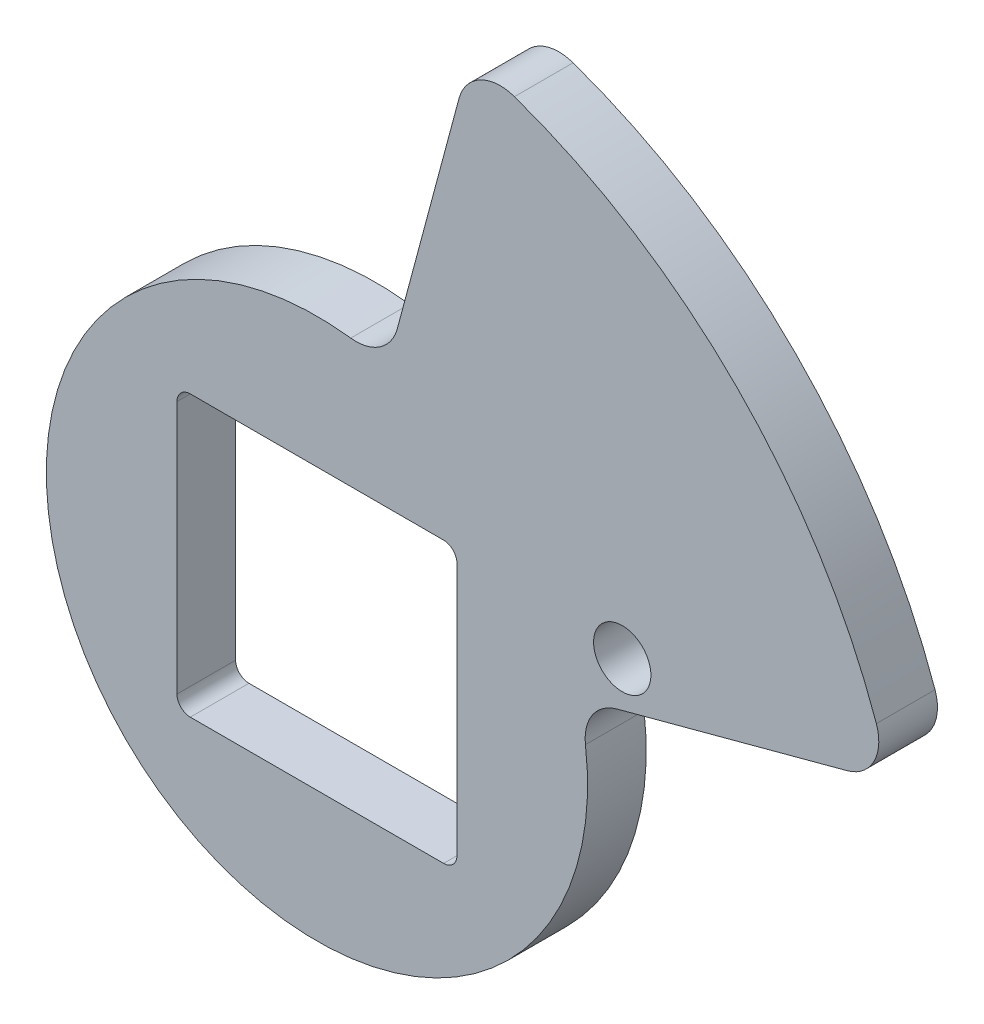
ISO-10303-21;
HEADER;
FILE_DESCRIPTION(('STEP AP214'),'2;1');
FILE_NAME('part.step','',(''),(''),'','','');
FILE_SCHEMA(('AUTOMOTIVE_DESIGN { 1 0 10303 214 1 1 1 1 }'));
ENDSEC;
DATA;
#1=APPLICATION_CONTEXT('core data for automotive mechanical design processes');
#2=APPLICATION_PROTOCOL_DEFINITION('international standard','automotive_design',2000,#1);
#3=PRODUCT_CONTEXT('',#1,'mechanical');
#4=PRODUCT('Part','Part','',(#3));
#5=PRODUCT_RELATED_PRODUCT_CATEGORY('part','',(#4));
#6=PRODUCT_DEFINITION_FORMATION('','',#4);
#7=PRODUCT_DEFINITION_CONTEXT('part definition',#1,'design');
#8=PRODUCT_DEFINITION('design','',#6,#7);
#9=PRODUCT_DEFINITION_SHAPE('','',#8);
#10=(LENGTH_UNIT() NAMED_UNIT(*) SI_UNIT(.MILLI.,.METRE.));
#11=(NAMED_UNIT(*) PLANE_ANGLE_UNIT() SI_UNIT($,.RADIAN.));
#12=(NAMED_UNIT(*) SI_UNIT($,.STERADIAN.) SOLID_ANGLE_UNIT());
#13=UNCERTAINTY_MEASURE_WITH_UNIT(LENGTH_MEASURE(1.E-05),#10,'distance_accuracy_value','');
#14=(GEOMETRIC_REPRESENTATION_CONTEXT(3) GLOBAL_UNCERTAINTY_ASSIGNED_CONTEXT((#13)) GLOBAL_UNIT_ASSIGNED_CONTEXT((#10,
#11,#12)) REPRESENTATION_CONTEXT('',''));
#15=CARTESIAN_POINT('',(0.,0.,0.));
#16=DIRECTION('',(0.,0.,1.));
#17=DIRECTION('',(1.,0.,0.));
#18=AXIS2_PLACEMENT_3D('',#15,#16,#17);
#19=CARTESIAN_POINT('',(2.93463155457416,23.316044639666,4.4));
#20=DIRECTION('',(0.,0.,-1.));
#21=DIRECTION('',(-1.,0.,0.));
#22=AXIS2_PLACEMENT_3D('',#19,#20,#21);
#23=CYLINDRICAL_SURFACE('',#22,3.20000000000004);
#24=CARTESIAN_POINT('',(2.93463155457416,23.316044639666,0.));
#25=DIRECTION('',(0.,0.,-1.));
#26=DIRECTION('',(1.,0.,0.));
#27=AXIS2_PLACEMENT_3D('',#24,#25,#26);
#28=CIRCLE('',#27,3.20000000000004);
#29=CARTESIAN_POINT('',(6.02559419869927,22.487823695338,0.));
#30=VERTEX_POINT('',#29);
#31=CARTESIAN_POINT('',(2.53502215139811,20.1410938802221,0.));
#32=VERTEX_POINT('',#31);
#33=EDGE_CURVE('E224',#30,#32,#28,.T.);
#34=ORIENTED_EDGE('',*,*,#33,.T.);
#35=DIRECTION('',(0.,0.,-1.));
#36=VECTOR('',#35,1.);
#37=CARTESIAN_POINT('',(2.53502215139811,20.1410938802221,4.4));
#38=LINE('',#37,#36);
#39=CARTESIAN_POINT('',(2.53502215139811,20.1410938802221,4.4));
#40=VERTEX_POINT('',#39);
#41=EDGE_CURVE('E259',#40,#32,#38,.T.);
#42=ORIENTED_EDGE('',*,*,#41,.F.);
#43=CARTESIAN_POINT('',(2.93463155457416,23.316044639666,4.4));
#44=DIRECTION('',(0.,0.,-1.));
#45=DIRECTION('',(1.,0.,0.));
#46=AXIS2_PLACEMENT_3D('',#43,#44,#45);
#47=CIRCLE('',#46,3.20000000000004);
#48=CARTESIAN_POINT('',(6.02559419869927,22.487823695338,4.4));
#49=VERTEX_POINT('',#48);
#50=EDGE_CURVE('E204',#49,#40,#47,.T.);
#51=ORIENTED_EDGE('',*,*,#50,.F.);
#52=DIRECTION('',(0.,0.,-1.));
#53=VECTOR('',#52,1.);
#54=CARTESIAN_POINT('',(6.02559419869927,22.487823695338,4.4));
#55=LINE('',#54,#53);
#56=EDGE_CURVE('E225',#49,#30,#55,.T.);
#57=ORIENTED_EDGE('',*,*,#56,.T.);
#58=EDGE_LOOP('',(#34,#42,#51,#57));
#59=FACE_BOUND('',#58,.T.);
#60=ADVANCED_FACE('F39',(#59),#23,.F.);
#61=CARTESIAN_POINT('',(0.,0.,4.4));
#62=DIRECTION('',(0.,0.,-1.));
#63=DIRECTION('',(-1.,0.,0.));
#64=AXIS2_PLACEMENT_3D('',#61,#62,#63);
#65=CYLINDRICAL_SURFACE('',#64,20.3);
#66=CARTESIAN_POINT('',(0.,0.,0.));
#67=DIRECTION('',(0.,0.,1.));
#68=DIRECTION('',(1.,0.,0.));
#69=AXIS2_PLACEMENT_3D('',#66,#67,#68);
#70=CIRCLE('',#69,20.3);
#71=CARTESIAN_POINT('',(20.1410938802221,2.5350221513982,0.));
#72=VERTEX_POINT('',#71);
#73=EDGE_CURVE('E227',#32,#72,#70,.T.);
#74=ORIENTED_EDGE('',*,*,#73,.T.);
#75=DIRECTION('',(0.,0.,-1.));
#76=VECTOR('',#75,1.);
#77=CARTESIAN_POINT('',(20.1410938802221,2.5350221513982,4.4));
#78=LINE('',#77,#76);
#79=CARTESIAN_POINT('',(20.1410938802221,2.5350221513982,4.4));
#80=VERTEX_POINT('',#79);
#81=EDGE_CURVE('E258',#80,#72,#78,.T.);
#82=ORIENTED_EDGE('',*,*,#81,.F.);
#83=CARTESIAN_POINT('',(0.,0.,4.4));
#84=DIRECTION('',(0.,0.,1.));
#85=DIRECTION('',(1.,0.,0.));
#86=AXIS2_PLACEMENT_3D('',#83,#84,#85);
#87=CIRCLE('',#86,20.3);
#88=EDGE_CURVE('E210',#40,#80,#87,.T.);
#89=ORIENTED_EDGE('',*,*,#88,.F.);
#90=ORIENTED_EDGE('',*,*,#41,.T.);
#91=EDGE_LOOP('',(#74,#82,#89,#90));
#92=FACE_BOUND('',#91,.T.);
#93=ADVANCED_FACE('F311',(#92),#65,.T.);
#94=CARTESIAN_POINT('',(23.316044639666,2.93463155457426,4.4));
#95=DIRECTION('',(0.,0.,-1.));
#96=DIRECTION('',(-1.,0.,0.));
#97=AXIS2_PLACEMENT_3D('',#94,#95,#96);
#98=CYLINDRICAL_SURFACE('',#97,3.2);
#99=CARTESIAN_POINT('',(23.316044639666,2.93463155457426,0.));
#100=DIRECTION('',(0.,0.,-1.));
#101=DIRECTION('',(1.,0.,0.));
#102=AXIS2_PLACEMENT_3D('',#99,#100,#101);
#103=CIRCLE('',#102,3.2);
#104=CARTESIAN_POINT('',(22.4878236953379,6.02559419869928,0.));
#105=VERTEX_POINT('',#104);
#106=EDGE_CURVE('E229',#72,#105,#103,.T.);
#107=ORIENTED_EDGE('',*,*,#106,.T.);
#108=DIRECTION('',(0.,0.,-1.));
#109=VECTOR('',#108,1.);
#110=CARTESIAN_POINT('',(22.4878236953379,6.02559419869928,4.4));
#111=LINE('',#110,#109);
#112=CARTESIAN_POINT('',(22.4878236953379,6.02559419869928,4.4));
#113=VERTEX_POINT('',#112);
#114=EDGE_CURVE('E251',#113,#105,#111,.T.);
#115=ORIENTED_EDGE('',*,*,#114,.F.);
#116=CARTESIAN_POINT('',(23.316044639666,2.93463155457426,4.4));
#117=DIRECTION('',(0.,0.,-1.));
#118=DIRECTION('',(1.,0.,0.));
#119=AXIS2_PLACEMENT_3D('',#116,#117,#118);
#120=CIRCLE('',#119,3.2);
#121=EDGE_CURVE('E209',#80,#113,#120,.T.);
#122=ORIENTED_EDGE('',*,*,#121,.F.);
#123=ORIENTED_EDGE('',*,*,#81,.T.);
#124=EDGE_LOOP('',(#107,#115,#122,#123));
#125=FACE_BOUND('',#124,.T.);
#126=ADVANCED_FACE('F318',(#125),#98,.F.);
#127=CARTESIAN_POINT('',(22.4878236953379,6.02559419869928,4.4));
#128=DIRECTION('',(-0.258819045102526,0.965925826289067,0.));
#129=DIRECTION('',(-0.965925826289067,-0.258819045102526,0.));
#130=AXIS2_PLACEMENT_3D('',#127,#128,#129);
#131=PLANE('',#130);
#132=DIRECTION('',(0.965925826289067,0.258819045102526,0.));
#133=VECTOR('',#132,1.);
#134=CARTESIAN_POINT('',(22.4878236953379,6.02559419869928,0.));
#135=LINE('',#134,#133);
#136=CARTESIAN_POINT('',(39.7728096244553,10.6570922195897,0.));
#137=VERTEX_POINT('',#136);
#138=EDGE_CURVE('E228',#105,#137,#135,.T.);
#139=ORIENTED_EDGE('',*,*,#138,.T.);
#140=DIRECTION('',(0.,0.,-1.));
#141=VECTOR('',#140,1.);
#142=CARTESIAN_POINT('',(39.7728096244553,10.6570922195897,4.4));
#143=LINE('',#142,#141);
#144=CARTESIAN_POINT('',(39.7728096244553,10.6570922195897,4.4));
#145=VERTEX_POINT('',#144);
#146=EDGE_CURVE('E246',#145,#137,#143,.T.);
#147=ORIENTED_EDGE('',*,*,#146,.F.);
#148=DIRECTION('',(0.965925826289067,0.258819045102526,0.));
#149=VECTOR('',#148,1.);
#150=CARTESIAN_POINT('',(22.4878236953379,6.02559419869928,4.4));
#151=LINE('',#150,#149);
#152=EDGE_CURVE('E215',#113,#145,#151,.T.);
#153=ORIENTED_EDGE('',*,*,#152,.F.);
#154=ORIENTED_EDGE('',*,*,#114,.T.);
#155=EDGE_LOOP('',(#139,#147,#153,#154));
#156=FACE_BOUND('',#155,.T.);
#157=ADVANCED_FACE('F355',(#156),#131,.F.);
#158=CARTESIAN_POINT('',(38.9445886801272,13.7480548637146,4.4));
#159=DIRECTION('',(0.,0.,-1.));
#160=DIRECTION('',(-1.,0.,0.));
#161=AXIS2_PLACEMENT_3D('',#158,#159,#160);
#162=CYLINDRICAL_SURFACE('',#161,3.19999999999996);
#163=CARTESIAN_POINT('',(38.9445886801272,13.7480548637146,0.));
#164=DIRECTION('',(0.,0.,1.));
#165=DIRECTION('',(1.,0.,0.));
#166=AXIS2_PLACEMENT_3D('',#163,#164,#165);
#167=CIRCLE('',#166,3.19999999999996);
#168=CARTESIAN_POINT('',(41.9620870766504,14.8132794536393,0.));
#169=VERTEX_POINT('',#168);
#170=EDGE_CURVE('E235',#137,#169,#167,.T.);
#171=ORIENTED_EDGE('',*,*,#170,.T.);
#172=DIRECTION('',(0.,0.,-1.));
#173=VECTOR('',#172,1.);
#174=CARTESIAN_POINT('',(41.9620870766504,14.8132794536393,4.4));
#175=LINE('',#174,#173);
#176=CARTESIAN_POINT('',(41.9620870766504,14.8132794536393,4.4));
#177=VERTEX_POINT('',#176);
#178=EDGE_CURVE('E250',#177,#169,#175,.T.);
#179=ORIENTED_EDGE('',*,*,#178,.F.);
#180=CARTESIAN_POINT('',(38.9445886801272,13.7480548637146,4.4));
#181=DIRECTION('',(0.,0.,1.));
#182=DIRECTION('',(1.,0.,0.));
#183=AXIS2_PLACEMENT_3D('',#180,#181,#182);
#184=CIRCLE('',#183,3.19999999999996);
#185=EDGE_CURVE('E212',#145,#177,#184,.T.);
#186=ORIENTED_EDGE('',*,*,#185,.F.);
#187=ORIENTED_EDGE('',*,*,#146,.T.);
#188=EDGE_LOOP('',(#171,#179,#186,#187));
#189=FACE_BOUND('',#188,.T.);
#190=ADVANCED_FACE('F346',(#189),#162,.T.);
#191=CARTESIAN_POINT('',(0.,0.,4.4));
#192=DIRECTION('',(0.,0.,-1.));
#193=DIRECTION('',(-1.,0.,0.));
#194=AXIS2_PLACEMENT_3D('',#191,#192,#193);
#195=CYLINDRICAL_SURFACE('',#194,44.5);
#196=CARTESIAN_POINT('',(0.,0.,0.));
#197=DIRECTION('',(0.,0.,1.));
#198=DIRECTION('',(1.,0.,0.));
#199=AXIS2_PLACEMENT_3D('',#196,#197,#198);
#200=CIRCLE('',#199,44.5);
#201=CARTESIAN_POINT('',(14.8132794536391,41.9620870766505,0.));
#202=VERTEX_POINT('',#201);
#203=EDGE_CURVE('E234',#169,#202,#200,.T.);
#204=ORIENTED_EDGE('',*,*,#203,.T.);
#205=DIRECTION('',(0.,0.,-1.));
#206=VECTOR('',#205,1.);
#207=CARTESIAN_POINT('',(14.8132794536391,41.9620870766505,4.4));
#208=LINE('',#207,#206);
#209=CARTESIAN_POINT('',(14.8132794536391,41.9620870766505,4.4));
#210=VERTEX_POINT('',#209);
#211=EDGE_CURVE('E241',#210,#202,#208,.T.);
#212=ORIENTED_EDGE('',*,*,#211,.F.);
#213=CARTESIAN_POINT('',(0.,0.,4.4));
#214=DIRECTION('',(0.,0.,1.));
#215=DIRECTION('',(1.,0.,0.));
#216=AXIS2_PLACEMENT_3D('',#213,#214,#215);
#217=CIRCLE('',#216,44.5);
#218=EDGE_CURVE('E216',#177,#210,#217,.T.);
#219=ORIENTED_EDGE('',*,*,#218,.F.);
#220=ORIENTED_EDGE('',*,*,#178,.T.);
#221=EDGE_LOOP('',(#204,#212,#219,#220));
#222=FACE_BOUND('',#221,.T.);
#223=ADVANCED_FACE('F343',(#222),#195,.T.);
#224=CARTESIAN_POINT('',(13.7480548637145,38.9445886801273,4.4));
#225=DIRECTION('',(0.,0.,-1.));
#226=DIRECTION('',(-1.,0.,0.));
#227=AXIS2_PLACEMENT_3D('',#224,#225,#226);
#228=CYLINDRICAL_SURFACE('',#227,3.2);
#229=CARTESIAN_POINT('',(13.7480548637145,38.9445886801273,0.));
#230=DIRECTION('',(0.,0.,1.));
#231=DIRECTION('',(1.,0.,0.));
#232=AXIS2_PLACEMENT_3D('',#229,#230,#231);
#233=CIRCLE('',#232,3.2);
#234=CARTESIAN_POINT('',(10.6570922195894,39.7728096244553,0.));
#235=VERTEX_POINT('',#234);
#236=EDGE_CURVE('E237',#202,#235,#233,.T.);
#237=ORIENTED_EDGE('',*,*,#236,.T.);
#238=DIRECTION('',(0.,0.,-1.));
#239=VECTOR('',#238,1.);
#240=CARTESIAN_POINT('',(10.6570922195894,39.7728096244553,4.4));
#241=LINE('',#240,#239);
#242=CARTESIAN_POINT('',(10.6570922195894,39.7728096244553,4.4));
#243=VERTEX_POINT('',#242);
#244=EDGE_CURVE('E242',#243,#235,#241,.T.);
#245=ORIENTED_EDGE('',*,*,#244,.F.);
#246=CARTESIAN_POINT('',(13.7480548637145,38.9445886801273,4.4));
#247=DIRECTION('',(0.,0.,1.));
#248=DIRECTION('',(1.,0.,0.));
#249=AXIS2_PLACEMENT_3D('',#246,#247,#248);
#250=CIRCLE('',#249,3.2);
#251=EDGE_CURVE('E217',#210,#243,#250,.T.);
#252=ORIENTED_EDGE('',*,*,#251,.F.);
#253=ORIENTED_EDGE('',*,*,#211,.T.);
#254=EDGE_LOOP('',(#237,#245,#252,#253));
#255=FACE_BOUND('',#254,.T.);
#256=ADVANCED_FACE('F339',(#255),#228,.T.);
#257=CARTESIAN_POINT('',(6.02559419869927,22.487823695338,4.4));
#258=DIRECTION('',(0.96592582628907,-0.258819045102513,0.));
#259=DIRECTION('',(0.258819045102513,0.96592582628907,0.));
#260=AXIS2_PLACEMENT_3D('',#257,#258,#259);
#261=PLANE('',#260);
#262=DIRECTION('',(-0.258819045102513,-0.96592582628907,0.));
#263=VECTOR('',#262,1.);
#264=CARTESIAN_POINT('',(6.02559419869927,22.487823695338,0.));
#265=LINE('',#264,#263);
#266=EDGE_CURVE('E208',#235,#30,#265,.T.);
#267=ORIENTED_EDGE('',*,*,#266,.T.);
#268=ORIENTED_EDGE('',*,*,#56,.F.);
#269=DIRECTION('',(-0.258819045102513,-0.96592582628907,0.));
#270=VECTOR('',#269,1.);
#271=CARTESIAN_POINT('',(6.02559419869927,22.487823695338,4.4));
#272=LINE('',#271,#270);
#273=EDGE_CURVE('E219',#243,#49,#272,.T.);
#274=ORIENTED_EDGE('',*,*,#273,.F.);
#275=ORIENTED_EDGE('',*,*,#244,.T.);
#276=EDGE_LOOP('',(#267,#268,#274,#275));
#277=FACE_BOUND('',#276,.T.);
#278=ADVANCED_FACE('F337',(#277),#261,.F.);
#279=CARTESIAN_POINT('',(2.93463155457416,23.316044639666,4.4));
#280=DIRECTION('',(0.,0.,1.));
#281=DIRECTION('',(1.,0.,0.));
#282=AXIS2_PLACEMENT_3D('',#279,#280,#281);
#283=PLANE('',#282);
#284=CARTESIAN_POINT('',(-9.5,-9.5,4.4));
#285=DIRECTION('',(0.,0.,1.));
#286=DIRECTION('',(1.,0.,0.));
#287=AXIS2_PLACEMENT_3D('',#284,#285,#286);
#288=CIRCLE('',#287,0.999999999999999);
#289=CARTESIAN_POINT('',(-10.5,-9.49999999999999,4.4));
#290=VERTEX_POINT('',#289);
#291=CARTESIAN_POINT('',(-9.49999999999999,-10.5,4.4));
#292=VERTEX_POINT('',#291);
#293=EDGE_CURVE('E52',#290,#292,#288,.T.);
#294=ORIENTED_EDGE('',*,*,#293,.F.);
#295=DIRECTION('',(0.,-1.,0.));
#296=VECTOR('',#295,1.);
#297=CARTESIAN_POINT('',(-10.5,0.,4.4));
#298=LINE('',#297,#296);
#299=CARTESIAN_POINT('',(-10.5,9.49999999999999,4.4));
#300=VERTEX_POINT('',#299);
#301=EDGE_CURVE('E183',#300,#290,#298,.T.);
#302=ORIENTED_EDGE('',*,*,#301,.F.);
#303=CARTESIAN_POINT('',(-9.5,9.5,4.4));
#304=DIRECTION('',(0.,0.,1.));
#305=DIRECTION('',(1.,0.,0.));
#306=AXIS2_PLACEMENT_3D('',#303,#304,#305);
#307=CIRCLE('',#306,0.999999999999999);
#308=CARTESIAN_POINT('',(-9.49999999999999,10.5,4.4));
#309=VERTEX_POINT('',#308);
#310=EDGE_CURVE('E185',#309,#300,#307,.T.);
#311=ORIENTED_EDGE('',*,*,#310,.F.);
#312=DIRECTION('',(-1.,0.,0.));
#313=VECTOR('',#312,1.);
#314=CARTESIAN_POINT('',(9.49999999999999,10.5,4.4));
#315=LINE('',#314,#313);
#316=CARTESIAN_POINT('',(9.49999999999999,10.5,4.4));
#317=VERTEX_POINT('',#316);
#318=EDGE_CURVE('E179',#317,#309,#315,.T.);
#319=ORIENTED_EDGE('',*,*,#318,.F.);
#320=CARTESIAN_POINT('',(9.5,9.5,4.4));
#321=DIRECTION('',(0.,0.,1.));
#322=DIRECTION('',(1.,0.,0.));
#323=AXIS2_PLACEMENT_3D('',#320,#321,#322);
#324=CIRCLE('',#323,0.999999999999999);
#325=CARTESIAN_POINT('',(10.5,9.49999999999999,4.4));
#326=VERTEX_POINT('',#325);
#327=EDGE_CURVE('E174',#326,#317,#324,.T.);
#328=ORIENTED_EDGE('',*,*,#327,.F.);
#329=DIRECTION('',(0.,1.,0.));
#330=VECTOR('',#329,1.);
#331=CARTESIAN_POINT('',(10.5,-9.49999999999999,4.4));
#332=LINE('',#331,#330);
#333=CARTESIAN_POINT('',(10.5,-9.49999999999999,4.4));
#334=VERTEX_POINT('',#333);
#335=EDGE_CURVE('E172',#334,#326,#332,.T.);
#336=ORIENTED_EDGE('',*,*,#335,.F.);
#337=CARTESIAN_POINT('',(9.5,-9.5,4.4));
#338=DIRECTION('',(0.,0.,1.));
#339=DIRECTION('',(1.,0.,0.));
#340=AXIS2_PLACEMENT_3D('',#337,#338,#339);
#341=CIRCLE('',#340,1.);
#342=CARTESIAN_POINT('',(9.49999999999999,-10.5,4.4));
#343=VERTEX_POINT('',#342);
#344=EDGE_CURVE('E152',#343,#334,#341,.T.);
#345=ORIENTED_EDGE('',*,*,#344,.F.);
#346=DIRECTION('',(1.,0.,0.));
#347=VECTOR('',#346,1.);
#348=CARTESIAN_POINT('',(-9.49999999999999,-10.5,4.4));
#349=LINE('',#348,#347);
#350=EDGE_CURVE('E162',#292,#343,#349,.T.);
#351=ORIENTED_EDGE('',*,*,#350,.F.);
#352=EDGE_LOOP('',(#294,#302,#311,#319,#328,#336,#345,#351));
#353=FACE_BOUND('',#352,.T.);
#354=CARTESIAN_POINT('',(22.9,9.5,4.4));
#355=DIRECTION('',(0.,0.,1.));
#356=DIRECTION('',(1.,0.,0.));
#357=AXIS2_PLACEMENT_3D('',#354,#355,#356);
#358=CIRCLE('',#357,2.15);
#359=CARTESIAN_POINT('',(25.05,9.5,4.4));
#360=VERTEX_POINT('',#359);
#361=EDGE_CURVE('E203',#360,#360,#358,.T.);
#362=ORIENTED_EDGE('',*,*,#361,.F.);
#363=EDGE_LOOP('',(#362));
#364=FACE_BOUND('',#363,.T.);
#365=ORIENTED_EDGE('',*,*,#50,.T.);
#366=ORIENTED_EDGE('',*,*,#88,.T.);
#367=ORIENTED_EDGE('',*,*,#121,.T.);
#368=ORIENTED_EDGE('',*,*,#152,.T.);
#369=ORIENTED_EDGE('',*,*,#185,.T.);
#370=ORIENTED_EDGE('',*,*,#218,.T.);
#371=ORIENTED_EDGE('',*,*,#251,.T.);
#372=ORIENTED_EDGE('',*,*,#273,.T.);
#373=EDGE_LOOP('',(#365,#366,#367,#368,#369,#370,#371,#372));
#374=FACE_BOUND('',#373,.T.);
#375=ADVANCED_FACE('F170',(#353,#364,#374),#283,.T.);
#376=CARTESIAN_POINT('',(2.93463155457416,23.316044639666,0.));
#377=DIRECTION('',(0.,0.,1.));
#378=DIRECTION('',(1.,0.,0.));
#379=AXIS2_PLACEMENT_3D('',#376,#377,#378);
#380=PLANE('',#379);
#381=DIRECTION('',(0.,-1.,0.));
#382=VECTOR('',#381,1.);
#383=CARTESIAN_POINT('',(-10.5,23.316044639666,0.));
#384=LINE('',#383,#382);
#385=CARTESIAN_POINT('',(-10.5,9.49999999999999,0.));
#386=VERTEX_POINT('',#385);
#387=CARTESIAN_POINT('',(-10.5,-9.49999999999999,0.));
#388=VERTEX_POINT('',#387);
#389=EDGE_CURVE('E46',#386,#388,#384,.T.);
#390=ORIENTED_EDGE('',*,*,#389,.T.);
#391=CARTESIAN_POINT('',(-9.5,-9.5,0.));
#392=DIRECTION('',(0.,0.,1.));
#393=DIRECTION('',(1.,0.,0.));
#394=AXIS2_PLACEMENT_3D('',#391,#392,#393);
#395=CIRCLE('',#394,0.999999999999999);
#396=CARTESIAN_POINT('',(-9.49999999999999,-10.5,0.));
#397=VERTEX_POINT('',#396);
#398=EDGE_CURVE('E11',#388,#397,#395,.T.);
#399=ORIENTED_EDGE('',*,*,#398,.T.);
#400=DIRECTION('',(1.,0.,0.));
#401=VECTOR('',#400,1.);
#402=CARTESIAN_POINT('',(2.93463155457416,-10.5,0.));
#403=LINE('',#402,#401);
#404=CARTESIAN_POINT('',(9.49999999999999,-10.5,0.));
#405=VERTEX_POINT('',#404);
#406=EDGE_CURVE('E265',#397,#405,#403,.T.);
#407=ORIENTED_EDGE('',*,*,#406,.T.);
#408=CARTESIAN_POINT('',(9.5,-9.5,0.));
#409=DIRECTION('',(0.,0.,1.));
#410=DIRECTION('',(1.,0.,0.));
#411=AXIS2_PLACEMENT_3D('',#408,#409,#410);
#412=CIRCLE('',#411,1.);
#413=CARTESIAN_POINT('',(10.5,-9.49999999999999,0.));
#414=VERTEX_POINT('',#413);
#415=EDGE_CURVE('E160',#405,#414,#412,.T.);
#416=ORIENTED_EDGE('',*,*,#415,.T.);
#417=DIRECTION('',(0.,1.,0.));
#418=VECTOR('',#417,1.);
#419=CARTESIAN_POINT('',(10.5,23.316044639666,0.));
#420=LINE('',#419,#418);
#421=CARTESIAN_POINT('',(10.5,9.49999999999999,0.));
#422=VERTEX_POINT('',#421);
#423=EDGE_CURVE('E270',#414,#422,#420,.T.);
#424=ORIENTED_EDGE('',*,*,#423,.T.);
#425=CARTESIAN_POINT('',(9.5,9.5,0.));
#426=DIRECTION('',(0.,0.,1.));
#427=DIRECTION('',(1.,0.,0.));
#428=AXIS2_PLACEMENT_3D('',#425,#426,#427);
#429=CIRCLE('',#428,0.999999999999999);
#430=CARTESIAN_POINT('',(9.49999999999999,10.5,0.));
#431=VERTEX_POINT('',#430);
#432=EDGE_CURVE('E269',#422,#431,#429,.T.);
#433=ORIENTED_EDGE('',*,*,#432,.T.);
#434=DIRECTION('',(-1.,0.,0.));
#435=VECTOR('',#434,1.);
#436=CARTESIAN_POINT('',(2.93463155457416,10.5,0.));
#437=LINE('',#436,#435);
#438=CARTESIAN_POINT('',(-9.49999999999999,10.5,0.));
#439=VERTEX_POINT('',#438);
#440=EDGE_CURVE('E272',#431,#439,#437,.T.);
#441=ORIENTED_EDGE('',*,*,#440,.T.);
#442=CARTESIAN_POINT('',(-9.5,9.5,0.));
#443=DIRECTION('',(0.,0.,1.));
#444=DIRECTION('',(1.,0.,0.));
#445=AXIS2_PLACEMENT_3D('',#442,#443,#444);
#446=CIRCLE('',#445,0.999999999999999);
#447=EDGE_CURVE('E277',#439,#386,#446,.T.);
#448=ORIENTED_EDGE('',*,*,#447,.T.);
#449=EDGE_LOOP('',(#390,#399,#407,#416,#424,#433,#441,#448));
#450=FACE_BOUND('',#449,.T.);
#451=CARTESIAN_POINT('',(22.9,9.5,0.));
#452=DIRECTION('',(0.,0.,1.));
#453=DIRECTION('',(1.,0.,0.));
#454=AXIS2_PLACEMENT_3D('',#451,#452,#453);
#455=CIRCLE('',#454,2.15);
#456=CARTESIAN_POINT('',(25.05,9.5,0.));
#457=VERTEX_POINT('',#456);
#458=EDGE_CURVE('E188',#457,#457,#455,.T.);
#459=ORIENTED_EDGE('',*,*,#458,.T.);
#460=EDGE_LOOP('',(#459));
#461=FACE_BOUND('',#460,.T.);
#462=ORIENTED_EDGE('',*,*,#33,.F.);
#463=ORIENTED_EDGE('',*,*,#266,.F.);
#464=ORIENTED_EDGE('',*,*,#236,.F.);
#465=ORIENTED_EDGE('',*,*,#203,.F.);
#466=ORIENTED_EDGE('',*,*,#170,.F.);
#467=ORIENTED_EDGE('',*,*,#138,.F.);
#468=ORIENTED_EDGE('',*,*,#106,.F.);
#469=ORIENTED_EDGE('',*,*,#73,.F.);
#470=EDGE_LOOP('',(#462,#463,#464,#465,#466,#467,#468,#469));
#471=FACE_BOUND('',#470,.T.);
#472=ADVANCED_FACE('F278',(#450,#461,#471),#380,.F.);
#473=CARTESIAN_POINT('',(22.9,9.5,-24.));
#474=DIRECTION('',(0.,0.,1.));
#475=DIRECTION('',(1.,0.,0.));
#476=AXIS2_PLACEMENT_3D('',#473,#474,#475);
#477=CYLINDRICAL_SURFACE('',#476,2.15);
#478=ORIENTED_EDGE('',*,*,#361,.T.);
#479=EDGE_LOOP('',(#478));
#480=FACE_BOUND('',#479,.T.);
#481=ORIENTED_EDGE('',*,*,#458,.F.);
#482=EDGE_LOOP('',(#481));
#483=FACE_BOUND('',#482,.T.);
#484=ADVANCED_FACE('F305',(#480,#483),#477,.F.);
#485=CARTESIAN_POINT('',(-9.5,-9.5,-24.));
#486=DIRECTION('',(0.,0.,1.));
#487=DIRECTION('',(1.,0.,0.));
#488=AXIS2_PLACEMENT_3D('',#485,#486,#487);
#489=CYLINDRICAL_SURFACE('',#488,0.999999999999999);
#490=DIRECTION('',(0.,0.,1.));
#491=VECTOR('',#490,1.);
#492=CARTESIAN_POINT('',(-10.5,-9.49999999999999,-24.));
#493=LINE('',#492,#491);
#494=EDGE_CURVE('E189',#388,#290,#493,.T.);
#495=ORIENTED_EDGE('',*,*,#494,.T.);
#496=ORIENTED_EDGE('',*,*,#293,.T.);
#497=DIRECTION('',(0.,0.,1.));
#498=VECTOR('',#497,1.);
#499=CARTESIAN_POINT('',(-9.49999999999999,-10.5,-24.));
#500=LINE('',#499,#498);
#501=EDGE_CURVE('E159',#397,#292,#500,.T.);
#502=ORIENTED_EDGE('',*,*,#501,.F.);
#503=ORIENTED_EDGE('',*,*,#398,.F.);
#504=EDGE_LOOP('',(#495,#496,#502,#503));
#505=FACE_BOUND('',#504,.T.);
#506=ADVANCED_FACE('F298',(#505),#489,.F.);
#507=CARTESIAN_POINT('',(-10.5,0.,-24.));
#508=DIRECTION('',(-1.,0.,0.));
#509=DIRECTION('',(0.,-1.,0.));
#510=AXIS2_PLACEMENT_3D('',#507,#508,#509);
#511=PLANE('',#510);
#512=DIRECTION('',(0.,0.,1.));
#513=VECTOR('',#512,1.);
#514=CARTESIAN_POINT('',(-10.5,9.49999999999999,-24.));
#515=LINE('',#514,#513);
#516=EDGE_CURVE('E192',#386,#300,#515,.T.);
#517=ORIENTED_EDGE('',*,*,#516,.T.);
#518=ORIENTED_EDGE('',*,*,#301,.T.);
#519=ORIENTED_EDGE('',*,*,#494,.F.);
#520=ORIENTED_EDGE('',*,*,#389,.F.);
#521=EDGE_LOOP('',(#517,#518,#519,#520));
#522=FACE_BOUND('',#521,.T.);
#523=ADVANCED_FACE('F283',(#522),#511,.F.);
#524=CARTESIAN_POINT('',(-9.5,9.5,-24.));
#525=DIRECTION('',(0.,0.,1.));
#526=DIRECTION('',(1.,0.,0.));
#527=AXIS2_PLACEMENT_3D('',#524,#525,#526);
#528=CYLINDRICAL_SURFACE('',#527,0.999999999999999);
#529=DIRECTION('',(0.,0.,1.));
#530=VECTOR('',#529,1.);
#531=CARTESIAN_POINT('',(-9.49999999999999,10.5,-24.));
#532=LINE('',#531,#530);
#533=EDGE_CURVE('E193',#439,#309,#532,.T.);
#534=ORIENTED_EDGE('',*,*,#533,.T.);
#535=ORIENTED_EDGE('',*,*,#310,.T.);
#536=ORIENTED_EDGE('',*,*,#516,.F.);
#537=ORIENTED_EDGE('',*,*,#447,.F.);
#538=EDGE_LOOP('',(#534,#535,#536,#537));
#539=FACE_BOUND('',#538,.T.);
#540=ADVANCED_FACE('F290',(#539),#528,.F.);
#541=CARTESIAN_POINT('',(9.49999999999999,10.5,-24.));
#542=DIRECTION('',(0.,1.,0.));
#543=DIRECTION('',(0.,0.,1.));
#544=AXIS2_PLACEMENT_3D('',#541,#542,#543);
#545=PLANE('',#544);
#546=DIRECTION('',(0.,0.,1.));
#547=VECTOR('',#546,1.);
#548=CARTESIAN_POINT('',(9.49999999999999,10.5,-24.));
#549=LINE('',#548,#547);
#550=EDGE_CURVE('E191',#431,#317,#549,.T.);
#551=ORIENTED_EDGE('',*,*,#550,.T.);
#552=ORIENTED_EDGE('',*,*,#318,.T.);
#553=ORIENTED_EDGE('',*,*,#533,.F.);
#554=ORIENTED_EDGE('',*,*,#440,.F.);
#555=EDGE_LOOP('',(#551,#552,#553,#554));
#556=FACE_BOUND('',#555,.T.);
#557=ADVANCED_FACE('F291',(#556),#545,.F.);
#558=CARTESIAN_POINT('',(9.5,9.5,-24.));
#559=DIRECTION('',(0.,0.,1.));
#560=DIRECTION('',(1.,0.,0.));
#561=AXIS2_PLACEMENT_3D('',#558,#559,#560);
#562=CYLINDRICAL_SURFACE('',#561,0.999999999999999);
#563=DIRECTION('',(0.,0.,1.));
#564=VECTOR('',#563,1.);
#565=CARTESIAN_POINT('',(10.5,9.49999999999999,-24.));
#566=LINE('',#565,#564);
#567=EDGE_CURVE('E197',#422,#326,#566,.T.);
#568=ORIENTED_EDGE('',*,*,#567,.T.);
#569=ORIENTED_EDGE('',*,*,#327,.T.);
#570=ORIENTED_EDGE('',*,*,#550,.F.);
#571=ORIENTED_EDGE('',*,*,#432,.F.);
#572=EDGE_LOOP('',(#568,#569,#570,#571));
#573=FACE_BOUND('',#572,.T.);
#574=ADVANCED_FACE('F297',(#573),#562,.F.);
#575=CARTESIAN_POINT('',(10.5,-9.49999999999999,-24.));
#576=DIRECTION('',(1.,0.,0.));
#577=DIRECTION('',(0.,0.,-1.));
#578=AXIS2_PLACEMENT_3D('',#575,#576,#577);
#579=PLANE('',#578);
#580=DIRECTION('',(0.,0.,1.));
#581=VECTOR('',#580,1.);
#582=CARTESIAN_POINT('',(10.5,-9.49999999999999,-24.));
#583=LINE('',#582,#581);
#584=EDGE_CURVE('E157',#414,#334,#583,.T.);
#585=ORIENTED_EDGE('',*,*,#584,.T.);
#586=ORIENTED_EDGE('',*,*,#335,.T.);
#587=ORIENTED_EDGE('',*,*,#567,.F.);
#588=ORIENTED_EDGE('',*,*,#423,.F.);
#589=EDGE_LOOP('',(#585,#586,#587,#588));
#590=FACE_BOUND('',#589,.T.);
#591=ADVANCED_FACE('F296',(#590),#579,.F.);
#592=CARTESIAN_POINT('',(9.5,-9.5,-24.));
#593=DIRECTION('',(0.,0.,1.));
#594=DIRECTION('',(1.,0.,0.));
#595=AXIS2_PLACEMENT_3D('',#592,#593,#594);
#596=CYLINDRICAL_SURFACE('',#595,1.);
#597=DIRECTION('',(0.,0.,1.));
#598=VECTOR('',#597,1.);
#599=CARTESIAN_POINT('',(9.49999999999999,-10.5,-24.));
#600=LINE('',#599,#598);
#601=EDGE_CURVE('E62',#405,#343,#600,.T.);
#602=ORIENTED_EDGE('',*,*,#601,.T.);
#603=ORIENTED_EDGE('',*,*,#344,.T.);
#604=ORIENTED_EDGE('',*,*,#584,.F.);
#605=ORIENTED_EDGE('',*,*,#415,.F.);
#606=EDGE_LOOP('',(#602,#603,#604,#605));
#607=FACE_BOUND('',#606,.T.);
#608=ADVANCED_FACE('F151',(#607),#596,.F.);
#609=CARTESIAN_POINT('',(-9.49999999999999,-10.5,-24.));
#610=DIRECTION('',(0.,-1.,0.));
#611=DIRECTION('',(0.,0.,-1.));
#612=AXIS2_PLACEMENT_3D('',#609,#610,#611);
#613=PLANE('',#612);
#614=ORIENTED_EDGE('',*,*,#501,.T.);
#615=ORIENTED_EDGE('',*,*,#350,.T.);
#616=ORIENTED_EDGE('',*,*,#601,.F.);
#617=ORIENTED_EDGE('',*,*,#406,.F.);
#618=EDGE_LOOP('',(#614,#615,#616,#617));
#619=FACE_BOUND('',#618,.T.);
#620=ADVANCED_FACE('F163',(#619),#613,.F.);
#621=CLOSED_SHELL('',(#60,#93,#126,#157,#190,#223,#256,#278,#375,#472,#484,#506,#523,#540,#557,
#574,#591,#608,#620));
#622=MANIFOLD_SOLID_BREP('B2',#621);
#623=ADVANCED_BREP_SHAPE_REPRESENTATION('',(#18,#622),#14);
#624=SHAPE_DEFINITION_REPRESENTATION(#9,#623);
ENDSEC;
END-ISO-10303-21;
